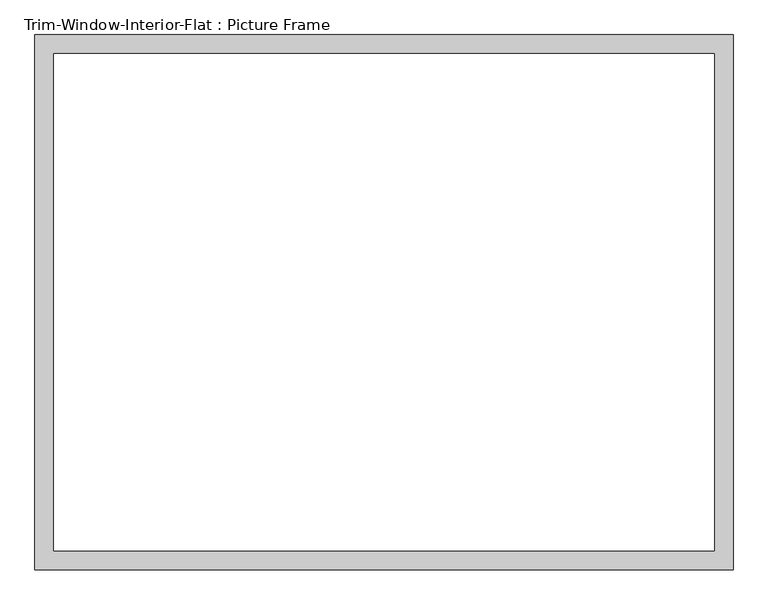
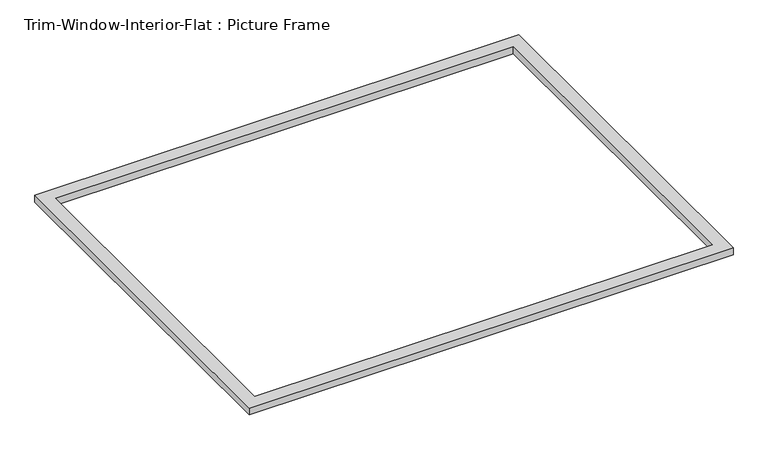
"""IFC4 building model written with IfcOpenShell, lengths in millimetres: proxy geometry, Trim-Window-Interior-Flat : Picture Frame."""

from ifc_helpers import new_model, si_unit, origin, origin_with_axes, place, context, project, spatial, polyline, outline, extrude, source, transform, mapped, element, save


def trim_window_interior_flat_picture_frame_fb3c0359(model_context):
    return source(origin(), model_context, "Body", "SweptSolid", [
        extrude(outline(polyline([(1051.6334769, 44.45), (1051.6334769, -1568.45), (-1051.6334769, -1568.45), (-1051.6334769, 44.45), (1051.6334769, 44.45)]), holes=[polyline([(994.4834769, -12.7), (-994.4834769, -12.7), (-994.4834769, -1511.3), (994.4834769, -1511.3), (994.4834769, -12.7)])]), origin_with_axes(), (0.0, 0.0, 1.0), 31.75),
    ])


if __name__ == "__main__":
    model = new_model("IFC4")
    model_context = context("Model", 3, world=origin())
    ifc_project = project(units=[si_unit("LENGTHUNIT", "METRE", prefix="MILLI")], contexts=[model_context])
    site = spatial("IfcSite", under=ifc_project)
    building = spatial("IfcBuilding", under=site)
    placement = place(None, origin())
    trim_window_interior_flat_picture_frame_shape = trim_window_interior_flat_picture_frame_fb3c0359(model_context)
    element("IfcBuildingElementProxy", 1, Name="Trim-Window-Interior-Flat : Picture Frame", ObjectType="Trim-Window-Interior-Flat : Picture Frame", at=placement, inside=building, context=model_context, shape_type="MappedRepresentation", body=[
        mapped(trim_window_interior_flat_picture_frame_shape, transform((0.0, 0.0, 0.0), x_axis=(1.0, 0.0, 0.0), y_axis=(0.0, 1.0, 0.0), z_axis=(0.0, 0.0, 1.0))),
    ])
    save(model, "model.ifc")

# Revit data of these elements
# Type "Trim-Window-Interior-Flat : Picture Frame"
#   Trim Thickness_Picture Frame = 0' - 1 1/4"
#   Trim Width = 0' - 2 1/4"
#   Trim Thickness_with Sill = 0' - 0 3/4"
#   Sill Thickness = 0' - 1 1/4"
#   Opening Width [instance default] = 2' - 0"
#   Opening Height [instance default] = 3' - 0"
#   Default Elevation = 4' - 0"
#   Sill = no
#   Picture Frame = yes
#   Trim Material [instance default] = none
# Element 1 (IfcBuildingElementProxy, "Trim-Window-Interior-Flat : Picture Frame")
#   Opening Width = 6' - 7.30579"
#   Opening Height = 5' - 0"
#   Trim Material = Wood - Stained
#   Materials on its faces: "Wood - Stained"
# Materials
#   "Wood - Stained": class "Wood", colour RGB 224 178 126, transparency 0, Cost = 0
